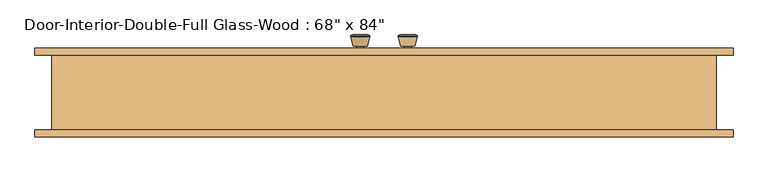
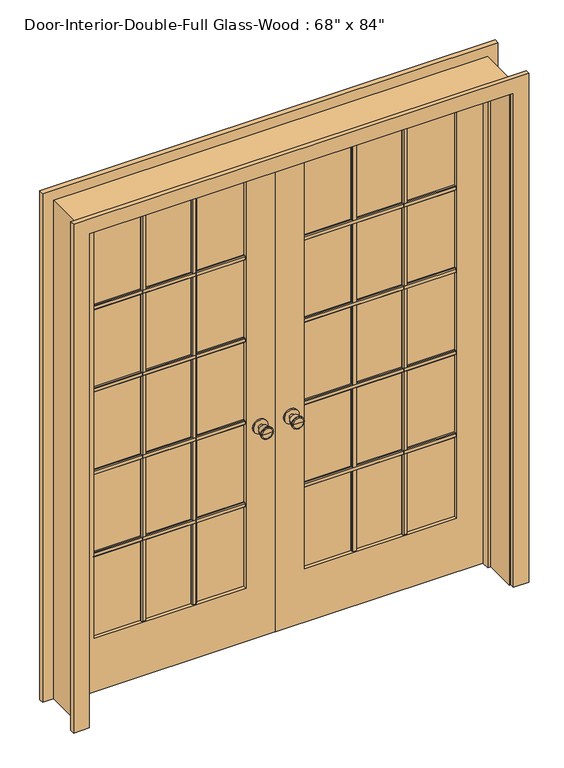
"""IFC4 building model written with IfcOpenShell, lengths in millimetres: door geometry."""

from ifc_helpers import new_model, si_unit, point, frame, frame_2d, origin, place, context, project, spatial, polyline, circle_curve, trimmed, segment, composite_curve, outline, extrude, faceted_brep, source, transform, mapped, element, save
from ifc_brep_helpers import plane_surface, cylinder_surface, revolved_surface, advanced_brep


def door_2f318157(model_context):
    return source(origin(), model_context, "Body", "SolidModel", [
        advanced_brep(
        [(-63.5, 102.825, 914.4), (-73.5, 102.825, 914.4), (-53.5, 102.825, 914.4), (-83.9758676, 151.825, 914.4), (-63.5, 151.825, 914.4), (-43.0241324, 151.825, 914.4), (-88.5, 149.9971319, 914.4), (-38.5, 149.9971319, 914.4), (-88.5, 146.5334537, 914.4), (-38.5, 146.5334537, 914.4), (-82.136236, 121.825, 914.4), (-44.863764, 121.825, 914.4), (-73.5, 121.825, 914.4), (-53.5, 121.825, 914.4)],
        [
            (0, 1),
            (1, 2, circle_curve(frame((-63.5, 102.825, 914.4), z_axis=(0.0, -1.0, 0.0), x_axis=(1.0, 0.0, 0.0)), 10.0)),
            (2, 0),
            (2, 1, circle_curve(frame((-63.5, 102.825, 914.4), z_axis=(0.0, -1.0, 0.0), x_axis=(1.0, 0.0, 0.0)), 10.0)),
            (3, 4),
            (4, 5),
            (5, 3, circle_curve(frame((-63.5, 151.825, 914.4), z_axis=(0.0, 1.0, 0.0), x_axis=(1.0, 0.0, 0.0)), 20.4758676)),
            (3, 5, circle_curve(frame((-63.5, 151.825, 914.4), z_axis=(0.0, 1.0, 0.0), x_axis=(1.0, 0.0, 0.0)), 20.4758676)),
            (6, 3),
            (5, 7),
            (7, 6, circle_curve(frame((-63.5, 149.9971319, 914.4), z_axis=(0.0, 1.0, 0.0), x_axis=(1.0, 0.0, 0.0)), 25.0)),
            (6, 7, circle_curve(frame((-63.5, 149.9971319, 914.4), z_axis=(0.0, 1.0, 0.0), x_axis=(1.0, 0.0, 0.0)), 25.0)),
            (8, 6),
            (7, 9),
            (9, 8, circle_curve(frame((-63.5, 146.5334537, 914.4), z_axis=(0.0, 1.0, 0.0), x_axis=(1.0, 0.0, 0.0)), 25.0)),
            (8, 9, circle_curve(frame((-63.5, 146.5334537, 914.4), z_axis=(0.0, 1.0, 0.0), x_axis=(1.0, 0.0, 0.0)), 25.0)),
            (10, 8),
            (9, 11),
            (11, 10, circle_curve(frame((-63.5, 121.825, 914.4), z_axis=(0.0, 1.0, 0.0), x_axis=(1.0, 0.0, 0.0)), 18.636236)),
            (10, 11, circle_curve(frame((-63.5, 121.825, 914.4), z_axis=(0.0, 1.0, 0.0), x_axis=(1.0, 0.0, 0.0)), 18.636236)),
            (12, 10),
            (11, 13),
            (13, 12, circle_curve(frame((-63.5, 121.825, 914.4), z_axis=(0.0, 1.0, 0.0), x_axis=(1.0, 0.0, 0.0)), 10.0)),
            (12, 13, circle_curve(frame((-63.5, 121.825, 914.4), z_axis=(0.0, 1.0, 0.0), x_axis=(1.0, 0.0, 0.0)), 10.0)),
            (1, 12),
            (13, 2),
        ],
        [
            plane_surface(frame((-63.5, 102.825, 914.4), z_axis=(0.0, -1.0, 0.0), x_axis=(1.0, 0.0, 0.0))),
            plane_surface(frame((-63.5, 151.825, 914.4), z_axis=(0.0, 1.0, 0.0), x_axis=(1.0, 0.0, 0.0))),
            revolved_surface(polyline([(-43.0241324, 151.825, 914.4), (-38.5, 149.9971319, 914.4)]), (-63.5, 102.825, 914.4), (0.0, -1.0, 0.0)),
            cylinder_surface(frame((-63.5, 102.825, 914.4), z_axis=(0.0, -1.0, 0.0), x_axis=(1.0, 0.0, 0.0)), 25.0),
            revolved_surface(polyline([(-38.5, 146.5334537, 914.4), (-44.863764, 121.825, 914.4)]), (-63.5, 102.825, 914.4), (0.0, -1.0, 0.0)),
            plane_surface(frame((-63.5, 121.825, 914.4), z_axis=(0.0, -1.0, 0.0), x_axis=(1.0, 0.0, 0.0))),
            cylinder_surface(frame((-63.5, 102.825, 914.4), z_axis=(0.0, -1.0, 0.0), x_axis=(1.0, 0.0, 0.0)), 10.0),
        ],
        [
            (0, [[1, 2, 3]]),
            (0, [[-3, 4, -1]]),
            (1, [[5, 6, 7]]),
            (1, [[-6, -5, 8]]),
            (2, [[9, -7, 10, 11]]),
            (2, [[-10, -8, -9, 12]]),
            (3, [[13, -11, 14, 15]]),
            (3, [[-14, -12, -13, 16]]),
            (4, [[17, -15, 18, 19]]),
            (4, [[-18, -16, -17, 20]]),
            (5, [[21, -19, 22, 23]]),
            (5, [[-22, -20, -21, 24]]),
            (6, [[25, -23, 26, -2]]),
            (6, [[-26, -24, -25, -4]]),
        ],
    ),
        extrude(outline(composite_curve([segment(trimmed(circle_curve(frame_2d((914.4, -63.5)), 30.0), [point((914.4, -33.5))], [point((914.4, -93.5))], False, "CARTESIAN"), True, "CONTINUOUS"), segment(trimmed(circle_curve(frame_2d((914.4, -63.5)), 30.0), [point((914.4, -93.5))], [point((914.4, -33.5))], False, "CARTESIAN"), True, "CONTINUOUS")], self_intersect=False)), frame((0.0, 96.825, 0.0), z_axis=(0.0, 1.0, 0.0), x_axis=(0.0, 0.0, 1.0)), (0.0, 0.0, 1.0), 6.0),
        advanced_brep(
        [(-63.5, 55.9, 914.4), (-53.5, 55.9, 914.4), (-73.5, 55.9, 914.4), (-83.9758676, 6.9, 914.4), (-43.0241324, 6.9, 914.4), (-63.5, 6.9, 914.4), (-88.5, 8.7278681, 914.4), (-38.5, 8.7278681, 914.4), (-88.5, 12.1915463, 914.4), (-38.5, 12.1915463, 914.4), (-82.136236, 36.9, 914.4), (-44.863764, 36.9, 914.4), (-73.5, 36.9, 914.4), (-53.5, 36.9, 914.4)],
        [
            (0, 1),
            (1, 2, circle_curve(frame((-63.5, 55.9, 914.4), z_axis=(0.0, 1.0, 0.0), x_axis=(1.0, 0.0, 0.0)), 10.0)),
            (2, 0),
            (2, 1, circle_curve(frame((-63.5, 55.9, 914.4), z_axis=(0.0, 1.0, 0.0), x_axis=(1.0, 0.0, 0.0)), 10.0)),
            (3, 4, circle_curve(frame((-63.5, 6.9, 914.4), z_axis=(0.0, -1.0, 0.0), x_axis=(1.0, 0.0, 0.0)), 20.4758676)),
            (4, 5),
            (5, 3),
            (4, 3, circle_curve(frame((-63.5, 6.9, 914.4), z_axis=(0.0, -1.0, 0.0), x_axis=(1.0, 0.0, 0.0)), 20.4758676)),
            (6, 7, circle_curve(frame((-63.5, 8.7278681, 914.4), z_axis=(0.0, -1.0, 0.0), x_axis=(1.0, 0.0, 0.0)), 25.0)),
            (7, 4),
            (3, 6),
            (7, 6, circle_curve(frame((-63.5, 8.7278681, 914.4), z_axis=(0.0, -1.0, 0.0), x_axis=(1.0, 0.0, 0.0)), 25.0)),
            (8, 9, circle_curve(frame((-63.5, 12.1915463, 914.4), z_axis=(0.0, -1.0, 0.0), x_axis=(1.0, 0.0, 0.0)), 25.0)),
            (9, 7),
            (6, 8),
            (9, 8, circle_curve(frame((-63.5, 12.1915463, 914.4), z_axis=(0.0, -1.0, 0.0), x_axis=(1.0, 0.0, 0.0)), 25.0)),
            (10, 11, circle_curve(frame((-63.5, 36.9, 914.4), z_axis=(0.0, -1.0, 0.0), x_axis=(1.0, 0.0, 0.0)), 18.636236)),
            (11, 9),
            (8, 10),
            (11, 10, circle_curve(frame((-63.5, 36.9, 914.4), z_axis=(0.0, -1.0, 0.0), x_axis=(1.0, 0.0, 0.0)), 18.636236)),
            (12, 13, circle_curve(frame((-63.5, 36.9, 914.4), z_axis=(0.0, -1.0, 0.0), x_axis=(1.0, 0.0, 0.0)), 10.0)),
            (13, 11),
            (10, 12),
            (13, 12, circle_curve(frame((-63.5, 36.9, 914.4), z_axis=(0.0, -1.0, 0.0), x_axis=(1.0, 0.0, 0.0)), 10.0)),
            (1, 13),
            (12, 2),
        ],
        [
            plane_surface(frame((-63.5, 55.9, 914.4), z_axis=(0.0, 1.0, 0.0), x_axis=(1.0, 0.0, 0.0))),
            plane_surface(frame((-63.5, 6.9, 914.4), z_axis=(0.0, -1.0, 0.0), x_axis=(1.0, 0.0, 0.0))),
            revolved_surface(polyline([(-43.0241324, 6.9, 914.4), (-38.5, 8.7278681, 914.4)]), (-63.5, 55.9, 914.4), (0.0, 1.0, 0.0)),
            cylinder_surface(frame((-63.5, 55.9, 914.4), z_axis=(0.0, 1.0, 0.0), x_axis=(1.0, 0.0, 0.0)), 25.0),
            revolved_surface(polyline([(-38.5, 12.1915463, 914.4), (-44.863764, 36.9, 914.4)]), (-63.5, 55.9, 914.4), (0.0, 1.0, 0.0)),
            plane_surface(frame((-63.5, 36.9, 914.4), z_axis=(0.0, 1.0, 0.0), x_axis=(1.0, 0.0, 0.0))),
            cylinder_surface(frame((-63.5, 55.9, 914.4), z_axis=(0.0, 1.0, 0.0), x_axis=(1.0, 0.0, 0.0)), 10.0),
        ],
        [
            (0, [[1, 2, 3]]),
            (0, [[-3, 4, -1]]),
            (1, [[5, 6, 7]]),
            (1, [[8, -7, -6]]),
            (2, [[9, 10, -5, 11]]),
            (2, [[12, -11, -8, -10]]),
            (3, [[13, 14, -9, 15]]),
            (3, [[16, -15, -12, -14]]),
            (4, [[17, 18, -13, 19]]),
            (4, [[20, -19, -16, -18]]),
            (5, [[21, 22, -17, 23]]),
            (5, [[24, -23, -20, -22]]),
            (6, [[-2, 25, -21, 26]]),
            (6, [[-4, -26, -24, -25]]),
        ],
    ),
        extrude(outline(composite_curve([segment(trimmed(circle_curve(frame_2d((914.4, -63.5)), 30.0), [point((914.4, -33.5))], [point((914.4, -93.5))], False, "CARTESIAN"), True, "CONTINUOUS"), segment(trimmed(circle_curve(frame_2d((914.4, -63.5)), 30.0), [point((914.4, -93.5))], [point((914.4, -33.5))], False, "CARTESIAN"), True, "CONTINUOUS")], self_intersect=False)), frame((0.0, 55.9, 0.0), z_axis=(0.0, 1.0, 0.0), x_axis=(0.0, 0.0, 1.0)), (0.0, 0.0, 1.0), 6.0),
        extrude(outline(polyline([(75.87, 1667.51), (75.87, 1648.46), (69.52, 1648.46), (66.345, 1651.635), (66.345, 1664.335), (69.52, 1667.51), (75.87, 1667.51)])), frame((120.65, 0.0, 0.0), z_axis=(1.0, 0.0, 0.0), x_axis=(0.0, 1.0, 0.0)), (0.0, 0.0, 1.0), 622.3),
        extrude(outline(polyline([(75.87, 1310.9575), (75.87, 1291.9075), (69.52, 1291.9075), (66.345, 1295.0825), (66.345, 1307.7825), (69.52, 1310.9575), (75.87, 1310.9575)])), frame((120.65, 0.0, 0.0), z_axis=(1.0, 0.0, 0.0), x_axis=(0.0, 1.0, 0.0)), (0.0, 0.0, 1.0), 622.3),
        extrude(outline(polyline([(75.87, 954.405), (75.87, 935.355), (69.52, 935.355), (66.345, 938.53), (66.345, 951.23), (69.52, 954.405), (75.87, 954.405)])), frame((120.65, 0.0, 0.0), z_axis=(1.0, 0.0, 0.0), x_axis=(0.0, 1.0, 0.0)), (0.0, 0.0, 1.0), 622.3),
        extrude(outline(polyline([(75.87, 597.8525), (75.87, 578.8025), (69.52, 578.8025), (66.345, 581.9775), (66.345, 594.6775), (69.52, 597.8525), (75.87, 597.8525)])), frame((120.65, 0.0, 0.0), z_axis=(1.0, 0.0, 0.0), x_axis=(0.0, 1.0, 0.0)), (0.0, 0.0, 1.0), 622.3),
        extrude(outline(polyline([(525.9916667, 75.87), (545.0416667, 75.87), (545.0416667, 69.52), (541.8666667, 66.345), (529.1666667, 66.345), (525.9916667, 69.52), (525.9916667, 75.87)])), frame((0.0, 0.0, 231.775), z_axis=(0.0, 0.0, 1.0), x_axis=(1.0, 0.0, 0.0)), (0.0, 0.0, 1.0), 1782.7625),
        extrude(outline(polyline([(318.5583333, 75.87), (337.6083333, 75.87), (337.6083333, 69.52), (334.4333333, 66.345), (321.7333333, 66.345), (318.5583333, 69.52), (318.5583333, 75.87)])), frame((0.0, 0.0, 231.775), z_axis=(0.0, 0.0, 1.0), x_axis=(1.0, 0.0, 0.0)), (0.0, 0.0, 1.0), 1782.7625),
        extrude(outline(polyline([(82.855, 1667.51), (89.205, 1667.51), (92.38, 1664.335), (92.38, 1651.635), (89.205, 1648.46), (82.855, 1648.46), (82.855, 1667.51)])), frame((-742.95, 0.0, 0.0), z_axis=(1.0, 0.0, 0.0), x_axis=(0.0, 1.0, 0.0)), (0.0, 0.0, 1.0), 622.3),
        extrude(outline(polyline([(82.855, 1310.9575), (89.205, 1310.9575), (92.38, 1307.7825), (92.38, 1295.0825), (89.205, 1291.9075), (82.855, 1291.9075), (82.855, 1310.9575)])), frame((-742.95, 0.0, 0.0), z_axis=(1.0, 0.0, 0.0), x_axis=(0.0, 1.0, 0.0)), (0.0, 0.0, 1.0), 622.3),
        extrude(outline(polyline([(82.855, 954.405), (89.205, 954.405), (92.38, 951.23), (92.38, 938.53), (89.205, 935.355), (82.855, 935.355), (82.855, 954.405)])), frame((-742.95, 0.0, 0.0), z_axis=(1.0, 0.0, 0.0), x_axis=(0.0, 1.0, 0.0)), (0.0, 0.0, 1.0), 622.3),
        extrude(outline(polyline([(82.855, 597.8525), (89.205, 597.8525), (92.38, 594.6775), (92.38, 581.9775), (89.205, 578.8025), (82.855, 578.8025), (82.855, 597.8525)])), frame((-742.95, 0.0, 0.0), z_axis=(1.0, 0.0, 0.0), x_axis=(0.0, 1.0, 0.0)), (0.0, 0.0, 1.0), 622.3),
        extrude(outline(polyline([(-337.6083333, 82.855), (-337.6083333, 89.205), (-334.4333333, 92.38), (-321.7333333, 92.38), (-318.5583333, 89.205), (-318.5583333, 82.855), (-337.6083333, 82.855)])), frame((0.0, 0.0, 231.775), z_axis=(0.0, 0.0, 1.0), x_axis=(1.0, 0.0, 0.0)), (0.0, 0.0, 1.0), 1782.7625),
        extrude(outline(polyline([(-545.0416667, 82.855), (-545.0416667, 89.205), (-541.8666667, 92.38), (-529.1666667, 92.38), (-525.9916667, 89.205), (-525.9916667, 82.855), (-545.0416667, 82.855)])), frame((0.0, 0.0, 231.775), z_axis=(0.0, 0.0, 1.0), x_axis=(1.0, 0.0, 0.0)), (0.0, 0.0, 1.0), 1782.7625),
        extrude(outline(polyline([(82.855, 1667.51), (89.205, 1667.51), (92.38, 1664.335), (92.38, 1651.635), (89.205, 1648.46), (82.855, 1648.46), (82.855, 1667.51)])), frame((120.65, 0.0, 0.0), z_axis=(1.0, 0.0, 0.0), x_axis=(0.0, 1.0, 0.0)), (0.0, 0.0, 1.0), 622.3),
        extrude(outline(polyline([(82.855, 1310.9575), (89.205, 1310.9575), (92.38, 1307.7825), (92.38, 1295.0825), (89.205, 1291.9075), (82.855, 1291.9075), (82.855, 1310.9575)])), frame((120.65, 0.0, 0.0), z_axis=(1.0, 0.0, 0.0), x_axis=(0.0, 1.0, 0.0)), (0.0, 0.0, 1.0), 622.3),
        extrude(outline(polyline([(82.855, 954.405), (89.205, 954.405), (92.38, 951.23), (92.38, 938.53), (89.205, 935.355), (82.855, 935.355), (82.855, 954.405)])), frame((120.65, 0.0, 0.0), z_axis=(1.0, 0.0, 0.0), x_axis=(0.0, 1.0, 0.0)), (0.0, 0.0, 1.0), 622.3),
        extrude(outline(polyline([(82.855, 597.8525), (89.205, 597.8525), (92.38, 594.6775), (92.38, 581.9775), (89.205, 578.8025), (82.855, 578.8025), (82.855, 597.8525)])), frame((120.65, 0.0, 0.0), z_axis=(1.0, 0.0, 0.0), x_axis=(0.0, 1.0, 0.0)), (0.0, 0.0, 1.0), 622.3),
        extrude(outline(polyline([(525.9916667, 82.855), (525.9916667, 89.205), (529.1666667, 92.38), (541.8666667, 92.38), (545.0416667, 89.205), (545.0416667, 82.855), (525.9916667, 82.855)])), frame((0.0, 0.0, 231.775), z_axis=(0.0, 0.0, 1.0), x_axis=(1.0, 0.0, 0.0)), (0.0, 0.0, 1.0), 1782.7625),
        extrude(outline(polyline([(318.5583333, 82.855), (318.5583333, 89.205), (321.7333333, 92.38), (334.4333333, 92.38), (337.6083333, 89.205), (337.6083333, 82.855), (318.5583333, 82.855)])), frame((0.0, 0.0, 231.775), z_axis=(0.0, 0.0, 1.0), x_axis=(1.0, 0.0, 0.0)), (0.0, 0.0, 1.0), 1782.7625),
        extrude(outline(polyline([(75.87, 1667.51), (75.87, 1648.46), (69.52, 1648.46), (66.345, 1651.635), (66.345, 1664.335), (69.52, 1667.51), (75.87, 1667.51)])), frame((-742.95, 0.0, 0.0), z_axis=(1.0, 0.0, 0.0), x_axis=(0.0, 1.0, 0.0)), (0.0, 0.0, 1.0), 622.3),
        extrude(outline(polyline([(75.87, 1310.9575), (75.87, 1291.9075), (69.52, 1291.9075), (66.345, 1295.0825), (66.345, 1307.7825), (69.52, 1310.9575), (75.87, 1310.9575)])), frame((-742.95, 0.0, 0.0), z_axis=(1.0, 0.0, 0.0), x_axis=(0.0, 1.0, 0.0)), (0.0, 0.0, 1.0), 622.3),
        extrude(outline(polyline([(75.87, 954.405), (75.87, 935.355), (69.52, 935.355), (66.345, 938.53), (66.345, 951.23), (69.52, 954.405), (75.87, 954.405)])), frame((-742.95, 0.0, 0.0), z_axis=(1.0, 0.0, 0.0), x_axis=(0.0, 1.0, 0.0)), (0.0, 0.0, 1.0), 622.3),
        extrude(outline(polyline([(75.87, 597.8525), (75.87, 578.8025), (69.52, 578.8025), (66.345, 581.9775), (66.345, 594.6775), (69.52, 597.8525), (75.87, 597.8525)])), frame((-742.95, 0.0, 0.0), z_axis=(1.0, 0.0, 0.0), x_axis=(0.0, 1.0, 0.0)), (0.0, 0.0, 1.0), 622.3),
        extrude(outline(polyline([(-337.6083333, 75.87), (-318.5583333, 75.87), (-318.5583333, 69.52), (-321.7333333, 66.345), (-334.4333333, 66.345), (-337.6083333, 69.52), (-337.6083333, 75.87)])), frame((0.0, 0.0, 231.775), z_axis=(0.0, 0.0, 1.0), x_axis=(1.0, 0.0, 0.0)), (0.0, 0.0, 1.0), 1782.7625),
        extrude(outline(polyline([(-545.0416667, 75.87), (-525.9916667, 75.87), (-525.9916667, 69.52), (-529.1666667, 66.345), (-541.8666667, 66.345), (-545.0416667, 69.52), (-545.0416667, 75.87)])), frame((0.0, 0.0, 231.775), z_axis=(0.0, 0.0, 1.0), x_axis=(1.0, 0.0, 0.0)), (0.0, 0.0, 1.0), 1782.7625),
        advanced_brep(
        [(63.5, 55.9, 914.4), (73.5, 55.9, 914.4), (53.5, 55.9, 914.4), (83.9758676, 6.9, 914.4), (63.5, 6.9, 914.4), (43.0241324, 6.9, 914.4), (88.5, 8.7278681, 914.4), (38.5, 8.7278681, 914.4), (88.5, 12.1915463, 914.4), (38.5, 12.1915463, 914.4), (82.136236, 36.9, 914.4), (44.863764, 36.9, 914.4), (73.5, 36.9, 914.4), (53.5, 36.9, 914.4)],
        [
            (0, 1),
            (1, 2, circle_curve(frame((63.5, 55.9, 914.4), z_axis=(0.0, 1.0, 0.0), x_axis=(-1.0, 0.0, 0.0)), 10.0)),
            (2, 0),
            (2, 1, circle_curve(frame((63.5, 55.9, 914.4), z_axis=(0.0, 1.0, 0.0), x_axis=(-1.0, 0.0, 0.0)), 10.0)),
            (3, 4),
            (4, 5),
            (5, 3, circle_curve(frame((63.5, 6.9, 914.4), z_axis=(0.0, -1.0, 0.0), x_axis=(-1.0, 0.0, 0.0)), 20.4758676)),
            (3, 5, circle_curve(frame((63.5, 6.9, 914.4), z_axis=(0.0, -1.0, 0.0), x_axis=(-1.0, 0.0, 0.0)), 20.4758676)),
            (6, 3),
            (5, 7),
            (7, 6, circle_curve(frame((63.5, 8.7278681, 914.4), z_axis=(0.0, -1.0, 0.0), x_axis=(-1.0, 0.0, 0.0)), 25.0)),
            (6, 7, circle_curve(frame((63.5, 8.7278681, 914.4), z_axis=(0.0, -1.0, 0.0), x_axis=(-1.0, 0.0, 0.0)), 25.0)),
            (8, 6),
            (7, 9),
            (9, 8, circle_curve(frame((63.5, 12.1915463, 914.4), z_axis=(0.0, -1.0, 0.0), x_axis=(-1.0, 0.0, 0.0)), 25.0)),
            (8, 9, circle_curve(frame((63.5, 12.1915463, 914.4), z_axis=(0.0, -1.0, 0.0), x_axis=(-1.0, 0.0, 0.0)), 25.0)),
            (10, 8),
            (9, 11),
            (11, 10, circle_curve(frame((63.5, 36.9, 914.4), z_axis=(0.0, -1.0, 0.0), x_axis=(-1.0, 0.0, 0.0)), 18.636236)),
            (10, 11, circle_curve(frame((63.5, 36.9, 914.4), z_axis=(0.0, -1.0, 0.0), x_axis=(-1.0, 0.0, 0.0)), 18.636236)),
            (12, 10),
            (11, 13),
            (13, 12, circle_curve(frame((63.5, 36.9, 914.4), z_axis=(0.0, -1.0, 0.0), x_axis=(-1.0, 0.0, 0.0)), 10.0)),
            (12, 13, circle_curve(frame((63.5, 36.9, 914.4), z_axis=(0.0, -1.0, 0.0), x_axis=(-1.0, 0.0, 0.0)), 10.0)),
            (1, 12),
            (13, 2),
        ],
        [
            plane_surface(frame((63.5, 55.9, 914.4), z_axis=(0.0, 1.0, 0.0), x_axis=(-1.0, 0.0, 0.0))),
            plane_surface(frame((63.5, 6.9, 914.4), z_axis=(0.0, -1.0, 0.0), x_axis=(-1.0, 0.0, 0.0))),
            revolved_surface(polyline([(43.0241324, 6.9, 914.4), (38.5, 8.7278681, 914.4)]), (63.5, 55.9, 914.4), (0.0, 1.0, 0.0)),
            cylinder_surface(frame((63.5, 55.9, 914.4), z_axis=(0.0, 1.0, 0.0), x_axis=(-1.0, 0.0, 0.0)), 25.0),
            revolved_surface(polyline([(38.5, 12.1915463, 914.4), (44.863764, 36.9, 914.4)]), (63.5, 55.9, 914.4), (0.0, 1.0, 0.0)),
            plane_surface(frame((63.5, 36.9, 914.4), z_axis=(0.0, 1.0, 0.0), x_axis=(-1.0, 0.0, 0.0))),
            cylinder_surface(frame((63.5, 55.9, 914.4), z_axis=(0.0, 1.0, 0.0), x_axis=(-1.0, 0.0, 0.0)), 10.0),
        ],
        [
            (0, [[1, 2, 3]]),
            (0, [[-3, 4, -1]]),
            (1, [[5, 6, 7]]),
            (1, [[-6, -5, 8]]),
            (2, [[9, -7, 10, 11]]),
            (2, [[-10, -8, -9, 12]]),
            (3, [[13, -11, 14, 15]]),
            (3, [[-14, -12, -13, 16]]),
            (4, [[17, -15, 18, 19]]),
            (4, [[-18, -16, -17, 20]]),
            (5, [[21, -19, 22, 23]]),
            (5, [[-22, -20, -21, 24]]),
            (6, [[25, -23, 26, -2]]),
            (6, [[-26, -24, -25, -4]]),
        ],
    ),
        extrude(outline(composite_curve([segment(trimmed(circle_curve(frame_2d((914.4, 63.5)), 30.0), [point((914.4, 33.5))], [point((914.4, 93.5))], False, "CARTESIAN"), True, "CONTINUOUS"), segment(trimmed(circle_curve(frame_2d((914.4, 63.5)), 30.0), [point((914.4, 93.5))], [point((914.4, 33.5))], False, "CARTESIAN"), True, "CONTINUOUS")], self_intersect=False)), frame((0.0, 55.9, 0.0), z_axis=(0.0, 1.0, 0.0), x_axis=(0.0, 0.0, 1.0)), (0.0, 0.0, 1.0), 6.0),
        advanced_brep(
        [(63.5, 102.825, 914.4), (53.5, 102.825, 914.4), (73.5, 102.825, 914.4), (83.9758676, 151.825, 914.4), (43.0241324, 151.825, 914.4), (63.5, 151.825, 914.4), (88.5, 149.9971319, 914.4), (38.5, 149.9971319, 914.4), (88.5, 146.5334537, 914.4), (38.5, 146.5334537, 914.4), (82.136236, 121.825, 914.4), (44.863764, 121.825, 914.4), (73.5, 121.825, 914.4), (53.5, 121.825, 914.4)],
        [
            (0, 1),
            (1, 2, circle_curve(frame((63.5, 102.825, 914.4), z_axis=(0.0, -1.0, 0.0), x_axis=(-1.0, 0.0, 0.0)), 10.0)),
            (2, 0),
            (2, 1, circle_curve(frame((63.5, 102.825, 914.4), z_axis=(0.0, -1.0, 0.0), x_axis=(-1.0, 0.0, 0.0)), 10.0)),
            (3, 4, circle_curve(frame((63.5, 151.825, 914.4), z_axis=(0.0, 1.0, 0.0), x_axis=(-1.0, 0.0, 0.0)), 20.4758676)),
            (4, 5),
            (5, 3),
            (4, 3, circle_curve(frame((63.5, 151.825, 914.4), z_axis=(0.0, 1.0, 0.0), x_axis=(-1.0, 0.0, 0.0)), 20.4758676)),
            (6, 7, circle_curve(frame((63.5, 149.9971319, 914.4), z_axis=(0.0, 1.0, 0.0), x_axis=(-1.0, 0.0, 0.0)), 25.0)),
            (7, 4),
            (3, 6),
            (7, 6, circle_curve(frame((63.5, 149.9971319, 914.4), z_axis=(0.0, 1.0, 0.0), x_axis=(-1.0, 0.0, 0.0)), 25.0)),
            (8, 9, circle_curve(frame((63.5, 146.5334537, 914.4), z_axis=(0.0, 1.0, 0.0), x_axis=(-1.0, 0.0, 0.0)), 25.0)),
            (9, 7),
            (6, 8),
            (9, 8, circle_curve(frame((63.5, 146.5334537, 914.4), z_axis=(0.0, 1.0, 0.0), x_axis=(-1.0, 0.0, 0.0)), 25.0)),
            (10, 11, circle_curve(frame((63.5, 121.825, 914.4), z_axis=(0.0, 1.0, 0.0), x_axis=(-1.0, 0.0, 0.0)), 18.636236)),
            (11, 9),
            (8, 10),
            (11, 10, circle_curve(frame((63.5, 121.825, 914.4), z_axis=(0.0, 1.0, 0.0), x_axis=(-1.0, 0.0, 0.0)), 18.636236)),
            (12, 13, circle_curve(frame((63.5, 121.825, 914.4), z_axis=(0.0, 1.0, 0.0), x_axis=(-1.0, 0.0, 0.0)), 10.0)),
            (13, 11),
            (10, 12),
            (13, 12, circle_curve(frame((63.5, 121.825, 914.4), z_axis=(0.0, 1.0, 0.0), x_axis=(-1.0, 0.0, 0.0)), 10.0)),
            (1, 13),
            (12, 2),
        ],
        [
            plane_surface(frame((63.5, 102.825, 914.4), z_axis=(0.0, -1.0, 0.0), x_axis=(-1.0, 0.0, 0.0))),
            plane_surface(frame((63.5, 151.825, 914.4), z_axis=(0.0, 1.0, 0.0), x_axis=(-1.0, 0.0, 0.0))),
            revolved_surface(polyline([(43.0241324, 151.825, 914.4), (38.5, 149.9971319, 914.4)]), (63.5, 102.825, 914.4), (0.0, -1.0, 0.0)),
            cylinder_surface(frame((63.5, 102.825, 914.4), z_axis=(0.0, -1.0, 0.0), x_axis=(-1.0, 0.0, 0.0)), 25.0),
            revolved_surface(polyline([(38.5, 146.5334537, 914.4), (44.863764, 121.825, 914.4)]), (63.5, 102.825, 914.4), (0.0, -1.0, 0.0)),
            plane_surface(frame((63.5, 121.825, 914.4), z_axis=(0.0, -1.0, 0.0), x_axis=(-1.0, 0.0, 0.0))),
            cylinder_surface(frame((63.5, 102.825, 914.4), z_axis=(0.0, -1.0, 0.0), x_axis=(-1.0, 0.0, 0.0)), 10.0),
        ],
        [
            (0, [[1, 2, 3]]),
            (0, [[-3, 4, -1]]),
            (1, [[5, 6, 7]]),
            (1, [[8, -7, -6]]),
            (2, [[9, 10, -5, 11]]),
            (2, [[12, -11, -8, -10]]),
            (3, [[13, 14, -9, 15]]),
            (3, [[16, -15, -12, -14]]),
            (4, [[17, 18, -13, 19]]),
            (4, [[20, -19, -16, -18]]),
            (5, [[21, 22, -17, 23]]),
            (5, [[24, -23, -20, -22]]),
            (6, [[-2, 25, -21, 26]]),
            (6, [[-4, -26, -24, -25]]),
        ],
    ),
        extrude(outline(composite_curve([segment(trimmed(circle_curve(frame_2d((914.4, 63.5)), 30.0), [point((914.4, 33.5))], [point((914.4, 93.5))], False, "CARTESIAN"), True, "CONTINUOUS"), segment(trimmed(circle_curve(frame_2d((914.4, 63.5)), 30.0), [point((914.4, 93.5))], [point((914.4, 33.5))], False, "CARTESIAN"), True, "CONTINUOUS")], self_intersect=False)), frame((0.0, 96.825, 0.0), z_axis=(0.0, 1.0, 0.0), x_axis=(0.0, 0.0, 1.0)), (0.0, 0.0, 1.0), 6.0),
        extrude(outline(polyline([(0.0, 869.95), (0.0, 933.45), (2203.45, 933.45), (2203.45, -933.45), (0.0, -933.45), (0.0, -869.95), (2139.95, -869.95), (2139.95, 869.95), (0.0, 869.95)])), frame((0.0, 96.825, 0.0), z_axis=(0.0, 1.0, 0.0), x_axis=(0.0, 0.0, 1.0)), (0.0, 0.0, 1.0), 19.05),
        extrude(outline(polyline([(0.0, 869.95), (0.0, 933.45), (2203.45, 933.45), (2203.45, -933.45), (0.0, -933.45), (0.0, -869.95), (2139.95, -869.95), (2139.95, 869.95), (0.0, 869.95)])), frame((0.0, -122.225, 0.0), z_axis=(0.0, 1.0, 0.0), x_axis=(0.0, 0.0, 1.0)), (0.0, 0.0, 1.0), 19.05),
        extrude(outline(polyline([(2133.6, -863.6), (0.0, -863.6), (0.0, -1.6019111), (2133.6, -1.6019111), (2133.6, -863.6)]), holes=[polyline([(231.775, -742.95), (2014.5375, -742.95), (2014.5375, -120.65), (231.775, -120.65), (231.775, -742.95)])]), frame((0.0, 61.9, 0.0), z_axis=(0.0, 1.0, 0.0), x_axis=(0.0, 0.0, 1.0)), (0.0, 0.0, 1.0), 34.925),
        extrude(outline(polyline([(0.0, 863.6), (2133.6, 863.6), (2133.6, 1.5875), (0.0, 1.5875), (0.0, 863.6)]), holes=[polyline([(2014.5375, 120.65), (2014.5375, 742.95), (231.775, 742.95), (231.775, 120.65), (2014.5375, 120.65)])]), frame((0.0, 61.9, 0.0), z_axis=(0.0, 1.0, 0.0), x_axis=(0.0, 0.0, 1.0)), (0.0, 0.0, 1.0), 34.925),
        faceted_brep([(889.0, 96.825, 0.0), (889.0, -103.175, 0.0), (863.6, -103.175, 0.0), (863.6, 26.975, 0.0), (850.9, 26.975, 0.0), (850.9, 61.9, 0.0), (863.6, 61.9, 0.0), (863.6, 96.825, 0.0), (889.0, 96.825, 2159.0), (889.0, -103.175, 2159.0), (-889.0, -103.175, 2159.0), (-889.0, -103.175, 0.0), (-863.6, -103.175, 0.0), (-863.6, -103.175, 2133.6), (863.6, -103.175, 2133.6), (863.6, 26.975, 2133.6), (-863.6, 26.975, 2133.6), (-863.6, 26.975, 0.0), (-850.9, 26.975, 0.0), (-850.9, 26.975, 2120.9), (850.9, 26.975, 2120.9), (850.9, 61.9, 2120.9), (1.5875, 61.9, 2120.9), (-1.6019111, 61.9, 2120.9), (-850.9, 61.9, 2120.9), (-850.9, 61.9, 0.0), (-863.6, 61.9, 0.0), (-863.6, 61.9, 2133.6), (-1.6019111, 61.9, 2133.6), (1.5875, 61.9, 2133.6), (863.6, 61.9, 2133.6), (863.6, 96.825, 2133.6), (1.5875, 96.825, 2133.6), (-1.6019111, 96.825, 2133.6), (-863.6, 96.825, 2133.6), (-863.6, 96.825, 0.0), (-889.0, 96.825, 0.0), (-889.0, 96.825, 2159.0)], [[[0, 1, 2, 3, 4, 5, 6, 7]], [[1, 0, 8, 9]], [[2, 1, 9, 10, 11, 12, 13, 14]], [[3, 2, 14, 15]], [[4, 3, 15, 16, 17, 18, 19, 20]], [[5, 4, 20, 21]], [[6, 5, 21, 22, 23, 24, 25, 26, 27, 28, 29, 30]], [[7, 6, 30, 31]], [[0, 7, 31, 32, 33, 34, 35, 36, 37, 8]], [[9, 8, 37, 10]], [[14, 13, 16, 15]], [[20, 19, 24, 23, 22, 21]], [[31, 30, 29, 28, 27, 34, 33, 32]], [[12, 11, 36, 35, 26, 25, 18, 17]], [[11, 10, 37, 36]], [[13, 12, 17, 16]], [[19, 18, 25, 24]], [[27, 26, 35, 34]]]),
        extrude(outline(polyline([(742.95, 75.87), (120.65, 75.87), (120.65, 82.855), (742.95, 82.855), (742.95, 75.87)])), frame((0.0, 0.0, 231.775), z_axis=(0.0, 0.0, 1.0), x_axis=(1.0, 0.0, 0.0)), (0.0, 0.0, 1.0), 1782.7625),
        extrude(outline(polyline([(-120.65, 75.87), (-742.95, 75.87), (-742.95, 82.855), (-120.65, 82.855), (-120.65, 75.87)])), frame((0.0, 0.0, 231.775), z_axis=(0.0, 0.0, 1.0), x_axis=(1.0, 0.0, 0.0)), (0.0, 0.0, 1.0), 1782.7625),
    ])


if __name__ == "__main__":
    model = new_model("IFC4")
    model_context = context("Model", 3, world=origin())
    ifc_project = project(units=[si_unit("LENGTHUNIT", "METRE", prefix="MILLI")], contexts=[model_context])
    site = spatial("IfcSite", under=ifc_project)
    building = spatial("IfcBuilding", under=site)
    placement = place(None, origin())
    door_shape = door_2f318157(model_context)
    element("IfcDoor", 1, ObjectType="Door-Interior-Double-Full Glass-Wood : 68\" x 84\"", at=placement, inside=building, context=model_context, shape_type="MappedRepresentation", body=[
        mapped(door_shape, transform((0.0, 0.0, 0.0), x_axis=(1.0, 0.0, 0.0), y_axis=(0.0, 1.0, 0.0), z_axis=(0.0, 0.0, 1.0))),
    ])
    save(model, "model.ifc")

# Revit data of these elements
# Type "Door-Interior-Double-Full Glass-Wood : 68\" x 84\""
#   Type Mark = "40"
#   Assembly Code = "C1020300"
#   Analytic Construction = "French door, wood frame with single glass"
#   Top Rail = 119.063 mm
#   Thickness = 34.925 mm
#   Thermal Resistance (R) = 0.188367 (m²·K)/W
#   Swing Angle [instance default] = 90.00°
#   Stiles = 120.65 mm
#   Rough Width = 1778 mm
#   Rough Height = 2159 mm
#   Panel Width = 863.6 mm
#   Height = 2133.6 mm
#   Width = 1727.2 mm
#   Heat Transfer Coefficient (U) = 5.30918 W/(m²·K)
#   Bottom Rail = 231.775 mm
#   Show Grill [instance default] = yes
#   Trim Material = Cherry
#   Panel Material = Cherry
#   Frame Material = Cherry
#   Door Handle Material = Aluminum
#   Visual Light Transmittance = 0
#   Solar Heat Gain Coefficient = 0
#   Wall Closure = (empty or 0)
#   Function = (empty or 0)
# Element 1 (IfcDoor, "Door-Interior-Double-Full Glass-Wood : 68\" x 84\"")
#   Materials on its faces: "Cherry", "Aluminum", "Glass"
# Materials
#   "Cherry": class "Wood", colour RGB 226 177 128, transparency 0, Description = "Prunus Serotina", Cost = 0
#   "Aluminum": class "Metal", colour RGB 247 247 247, transparency 0, Description = "Aluminum 6061", Cost = 0
#   "Glass": class "Glass", colour RGB 0 128 192, transparency 0.9, Description = "Soda Lime Glass", Cost = 0
